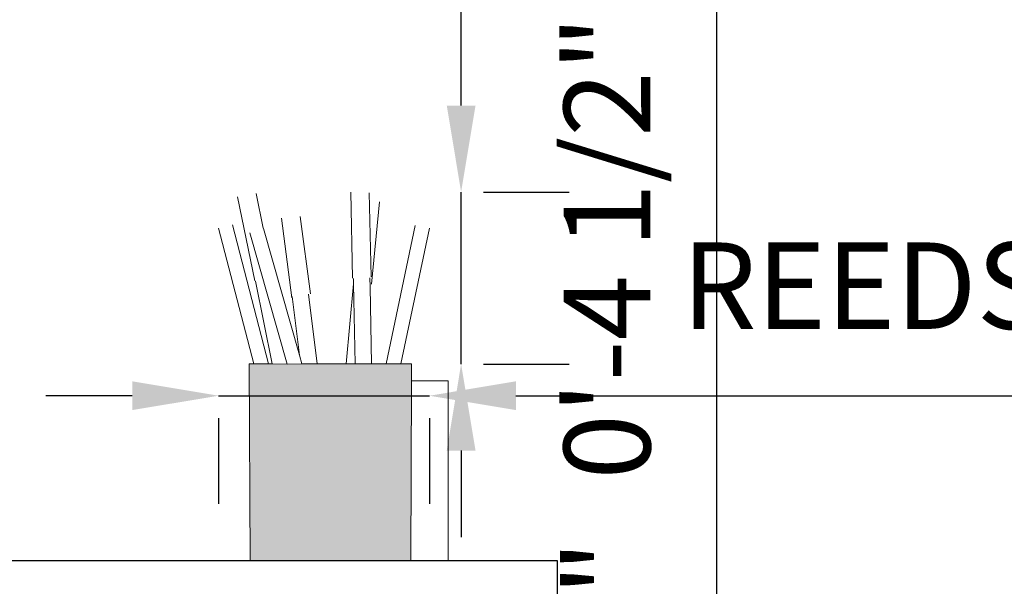
# Model space of a CAD drawing. Units: millimetres. Extents: x 7894 to 8038, y 6851 to 6951.
# Tile 14 of 49: x 7974.62 to 7986.01, y 6878.78 to 6885.34. Entities that reach past the tile are written whole.
import ezdxf

# ---------------------------------------------------------------- set-up
doc = ezdxf.new("R2010")
doc.units = ezdxf.units.MM
for name, color, linetype, lineweight in [('A-ANNO-DIMS', 2, 'Continuous', 18), ('A-FURN-ACCS', 8, 'Continuous', 13), ('A-FURN-SHLF', 7, 'Continuous', 30)]:
    doc.layers.add(name, color=color, linetype=linetype, lineweight=lineweight)
doc.layers.add('A-FURN-ACCS-PATT', color=116, linetype='Continuous', lineweight=9, true_color=0x136734)
doc.styles.get("Standard").update_dxf_attribs({"font": 'arial.ttf'})
doc.dimstyles.new('ISO-25', dxfattribs={"dimtxt": 1, "dimasz": 1, "dimexe": 1.25, "dimexo": 0.625, "dimtad": 1, "dimdec": 0, "dimlunit": 4, "dimtxsty": 'Standard', "dimcen": 2.5, "dimclrt": 1, "dimadec": 0, "dimazin": 0, "dimtfac": 1, "dimtdec": 0, "dimtmove": 0, "dimatfit": 3, "dimfxl": 1, "dimarcsym": 0})

# ---------------------------------------------------------------- blocks, each defined once
blk = doc.blocks.new('DISPLAY-REED-SPRAY')
for p, q in [((0.515, 1.573), (0.435, 1.972)), ((1.548, 0.994), (1.529, 1.989)), ((1.766, 1.01), (1.742, 1.98)), ((0.218, 1.934), (0.42, 0.963)), ((1.77, 0.926), (1.861, 1.878)), ((0.578, 0.003), (0.162, 1.611)), ((0.846, 0.767), (0.729, 1.689)), ((1.062, 0.811), (0.945, 1.707)), ((1.938, 0.003), (2.275, 1.603)), ((0, 1.572), (0.406, 0.001)), ((0.792, 0), (0.361, 1.519)), ((0.935, 0.103), (0.519, 1.567)), ((2.108, 0.001), (2.44, 1.573)), ((0.62, 0.003), (0.428, 0.96)), ((1.477, 0.003), (1.56, 0.927)), ((1.56, 0.991), (1.561, 0.935)), ((1.56, 0.927), (1.561, 0.935)), ((1.56, 0.927), (1.58, 0.003)), ((1.753, 0.892), (1.751, 0.999)), ((1.753, 0.892), (1.755, 0.914)), ((1.139, 0.003), (1.042, 0.808)), ((1.771, 0.003), (1.753, 0.892)), ((0.935, 0.103), (0.852, 0.78)), ((0.963, 0.002), (0.935, 0.103))]:
    blk.add_line(p, q)
blk = doc.blocks.new('*D19')
at = {"layer": 'A-ANNO-DIMS', "color": 0, "lineweight": -2, "transparency": 16777216}
for p, q in [((7975.917, 6880.988), (7974.917, 6880.988)), ((7976.917, 6880.988), (7979.357, 6880.988)), ((7980.357, 6880.988), (7996.183, 6880.988)), ((7976.917, 6880.729), (7976.917, 6879.738)), ((7979.357, 6880.729), (7979.357, 6879.738))]:
    blk.add_line(p, q, dxfattribs=at)
at = {"layer": 'A-ANNO-DIMS', "color": 0, "transparency": 16777216}
for points in [[(7975.917, 6881.155), (7975.917, 6880.822), (7976.917, 6880.988)], [(7980.357, 6881.155), (7980.357, 6880.822), (7979.357, 6880.988)]]:
    blk.add_solid(points, dxfattribs=at)
at = {"layer": 'Defpoints', "color": 0, "transparency": 16777216}
for p in [(7976.917, 6881.354), (7979.357, 6881.354), (7979.357, 6880.988)]:
    blk.add_point(p, dxfattribs=at)
at = {"layer": 'A-ANNO-DIMS', "color": 1, "transparency": 16777216, "insert": (7988.77, 6882.131), "char_height": 1, "attachment_point": 5}
blk.add_mtext('REEDS 0\'-2 1/2" TYP.', dxfattribs=at)
blk = doc.blocks.new('*D20')
at = {"layer": 'A-ANNO-DIMS', "color": 0, "lineweight": -2, "transparency": 16777216}
for p, q in [((7979.723, 6884.344), (7979.723, 6892.689)), ((7979.723, 6881.354), (7979.723, 6883.344)), ((7979.982, 6883.344), (7980.973, 6883.344)), ((7979.982, 6881.354), (7980.973, 6881.354)), ((7979.723, 6880.354), (7979.723, 6879.354))]:
    blk.add_line(p, q, dxfattribs=at)
at = {"layer": 'A-ANNO-DIMS', "color": 0, "transparency": 16777216}
for points in [[(7979.557, 6884.344), (7979.89, 6884.344), (7979.723, 6883.344)], [(7979.557, 6880.354), (7979.89, 6880.354), (7979.723, 6881.354)]]:
    blk.add_solid(points, dxfattribs=at)
at = {"layer": 'Defpoints', "color": 0, "transparency": 16777216}
for p in [(7979.357, 6883.344), (7979.723, 6883.344), (7979.357, 6881.354)]:
    blk.add_point(p, dxfattribs=at)
at = {"layer": 'A-ANNO-DIMS', "color": 1, "transparency": 16777216, "insert": (7978.588, 6889.016), "char_height": 1, "attachment_point": 5, "rotation": 90}
blk.add_mtext('0\'-2" TYP.', dxfattribs=at)
blk = doc.blocks.new('*D39')
at = {"layer": 'A-ANNO-DIMS', "color": 0, "lineweight": -2, "transparency": 16777216}
for p, q in [((7982.683, 6874.858), (7982.683, 6879.766)), ((7964.157, 6873.858), (7983.933, 6873.858)), ((7982.683, 6872.903), (7982.683, 6873.858)), ((7981.461, 6872.903), (7983.933, 6872.903)), ((7982.683, 6871.903), (7982.683, 6870.903))]:
    blk.add_line(p, q, dxfattribs=at)
at = {"layer": 'A-ANNO-DIMS', "color": 0, "transparency": 16777216}
for points in [[(7982.517, 6874.858), (7982.85, 6874.858), (7982.683, 6873.858)], [(7982.517, 6871.903), (7982.85, 6871.903), (7982.683, 6872.903)]]:
    blk.add_solid(points, dxfattribs=at)
at = {"layer": 'Defpoints', "color": 0, "transparency": 16777216}
for p in [(7963.532, 6873.858), (7982.683, 6873.858), (7980.836, 6872.903)]:
    blk.add_point(p, dxfattribs=at)
at = {"layer": 'A-ANNO-DIMS', "color": 1, "transparency": 16777216, "insert": (7981.548, 6877.812), "char_height": 1, "attachment_point": 5, "rotation": 90}
blk.add_mtext('0\'-1"', dxfattribs=at)
blk = doc.blocks.new('*D40')
at = {"layer": 'A-ANNO-DIMS', "color": 0, "lineweight": -2, "transparency": 16777216}
for p, q in [((7982.683, 6878.584), (7982.683, 6885.822)), ((7981.461, 6878.584), (7983.933, 6878.584)), ((7982.683, 6874.858), (7982.683, 6877.584)), ((7964.157, 6873.858), (7983.933, 6873.858))]:
    blk.add_line(p, q, dxfattribs=at)
at = {"layer": 'A-ANNO-DIMS', "color": 0, "transparency": 16777216}
for points in [[(7982.517, 6877.584), (7982.85, 6877.584), (7982.683, 6878.584)], [(7982.517, 6874.858), (7982.85, 6874.858), (7982.683, 6873.858)]]:
    blk.add_solid(points, dxfattribs=at)
at = {"layer": 'Defpoints', "color": 0, "transparency": 16777216}
for p in [(7980.836, 6878.584), (7982.683, 6878.584), (7963.532, 6873.858)]:
    blk.add_point(p, dxfattribs=at)
at = {"layer": 'A-ANNO-DIMS', "color": 1, "transparency": 16777216, "insert": (7981.541, 6882.703), "char_height": 1, "attachment_point": 5, "rotation": 90}
blk.add_mtext('0\'-4 1/2"', dxfattribs=at)

msp = doc.modelspace()

# ---------------------------------------------------------------- hatches: boundary and pattern name
at = {"layer": 'A-FURN-ACCS-PATT'}
h = msp.add_hatch(color=256, dxfattribs=at)
h.dxf.hatch_style = 1
h.paths.add_polyline_path([(7966.481, 6880.843), (7965.643, 6880.843), (7965.524, 6880.843), (7964.733, 6880.843), (7964.733, 6879.084), (7966.481, 6879.084)])
h.paths.add_polyline_path([(7967.067, 6866.98), (7966.229, 6866.98), (7966.11, 6866.98), (7965.32, 6866.98), (7965.32, 6865.222), (7967.067, 6865.222)])
h.paths.add_polyline_path([(7979.013, 6867.08), (7979.013, 6867.278), (7978.976, 6867.275), (7978.89, 6867.276), (7978.719, 6867.278), (7978.553, 6867.278), (7978.362, 6867.278), (7978.259, 6867.277), (7977.921, 6867.278), (7977.745, 6867.278), (7977.574, 6867.275), (7977.402, 6867.278), (7977.36, 6867.278), (7977.188, 6867.276), (7977.135, 6867.272), (7977.146, 6865.222), (7979.007, 6865.222)])
h.paths.add_polyline_path([(7977.402, 6867.278), (7977.36, 6867.278), (7977.188, 6867.276), (7977.177, 6867.275), (7977.171, 6867.276), (7977.385, 6867.278)])
h.paths.add_polyline_path([(7979.148, 6881.159), (7979.149, 6881.358), (7979.111, 6881.355), (7979.025, 6881.356), (7978.855, 6881.357), (7978.689, 6881.358), (7978.498, 6881.358), (7978.394, 6881.357), (7978.056, 6881.357), (7977.881, 6881.357), (7977.71, 6881.354), (7977.537, 6881.358), (7977.496, 6881.358), (7977.323, 6881.356), (7977.271, 6881.352), (7977.283, 6879.084), (7979.142, 6879.084)])
h.paths.add_polyline_path([(7977.537, 6881.358), (7977.496, 6881.358), (7977.323, 6881.356), (7977.313, 6881.355), (7977.306, 6881.355), (7977.521, 6881.358)])

# ---------------------------------------------------------------- linework, layer by layer
at = {"layer": 'A-FURN-ACCS'}
for p, q in [((7977.283, 6879.082), (7977.271, 6881.358)), ((7977.271, 6881.358), (7977.313, 6881.355)), ((7977.323, 6881.356), (7977.313, 6881.355)), ((7977.496, 6881.358), (7977.323, 6881.356)), ((7977.537, 6881.358), (7977.496, 6881.358)), ((7977.71, 6881.354), (7977.537, 6881.358)), ((7977.881, 6881.357), (7977.71, 6881.354)), ((7978.056, 6881.357), (7977.881, 6881.357)), ((7978.394, 6881.357), (7978.056, 6881.357)), ((7978.498, 6881.358), (7978.394, 6881.357)), ((7978.689, 6881.358), (7978.498, 6881.358)), ((7978.855, 6881.357), (7978.689, 6881.358)), ((7979.025, 6881.356), (7978.855, 6881.357)), ((7979.111, 6881.355), (7979.025, 6881.356)), ((7979.149, 6881.358), (7979.111, 6881.355)), ((7979.148, 6881.159), (7979.149, 6881.358)), ((7979.142, 6879.082), (7979.148, 6881.159)), ((7979.148, 6881.159), (7979.575, 6881.159)), ((7979.575, 6881.159), (7979.575, 6879.082)), ((7977.357, 6879.082), (7977.283, 6879.082)), ((7977.357, 6879.082), (7977.455, 6879.082)), ((7977.455, 6879.082), (7977.456, 6879.082)), ((7979.142, 6879.082), (7977.456, 6879.082)), ((7979.575, 6879.082), (7979.142, 6879.082))]:
    msp.add_line(p, q, dxfattribs=at)
at = {"layer": 'A-FURN-SHLF'}
for p, q in [((7963.532, 6879.084, -3.5), (7980.836, 6879.084, -3.5)), ((7980.836, 6879.084, -3.5), (7980.836, 6878.584, -3.5))]:
    msp.add_line(p, q, dxfattribs=at)

# ---------------------------------------------------------------- block references
at = {"layer": 'A-FURN-ACCS'}
msp.add_blockref('DISPLAY-REED-SPRAY', (7976.917, 6881.354), dxfattribs=at)

# ---------------------------------------------------------------- dimensions: what is measured, and where the dimension line sits
at = {"layer": 'A-ANNO-DIMS'}
dim = msp.add_linear_dim(base=(7979.723, 6883.344), p1=(7979.357, 6881.354), p2=(7979.357, 6883.344), angle=90, text='<> TYP.', dimstyle='ISO-25', override={"dimdec": 1, "dimlfac": 1, "dimrnd": 0, "dimzin": 1, "dimdsep": 46, "dimlunit": 4, "dimfrac": 2}, dxfattribs=at)
dim.commit()
dim.dimension.update_dxf_attribs({"geometry": '*D20', "text_midpoint": (7978.588, 6889.016)})
for base, p1, p2, picture, middle in [((7982.683, 6878.584), (7963.532, 6873.858), (7980.836, 6878.584), '*D40', (7981.541, 6882.703)), ((7982.683, 6873.858), (7980.836, 6872.903), (7963.532, 6873.858), '*D39', (7981.548, 6877.812))]:
    dim = msp.add_linear_dim(base=base, p1=p1, p2=p2, angle=90, dimstyle='ISO-25', override={"dimdec": 1, "dimlfac": 1, "dimrnd": 0, "dimzin": 1, "dimdsep": 46, "dimlunit": 4, "dimfrac": 2}, dxfattribs=at)
    dim.commit()
    dim.dimension.update_dxf_attribs({"geometry": picture, "text_midpoint": middle})
dim = msp.add_linear_dim(base=(7979.357, 6880.988), p1=(7976.917, 6881.354), p2=(7979.357, 6881.354), text='REEDS <> TYP.', dimstyle='ISO-25', override={"dimdec": 1, "dimlfac": 1, "dimrnd": 0, "dimzin": 1, "dimdsep": 46, "dimlunit": 4, "dimfrac": 2}, dxfattribs=at)
dim.commit()
dim.dimension.update_dxf_attribs({"geometry": '*D19', "text_midpoint": (7988.77, 6882.131)})

doc.saveas('drawing.dxf')
